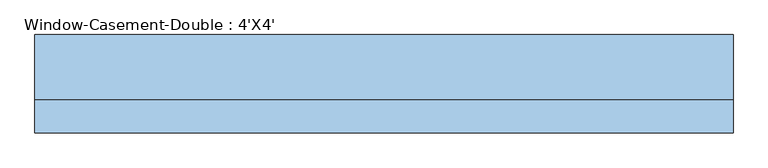
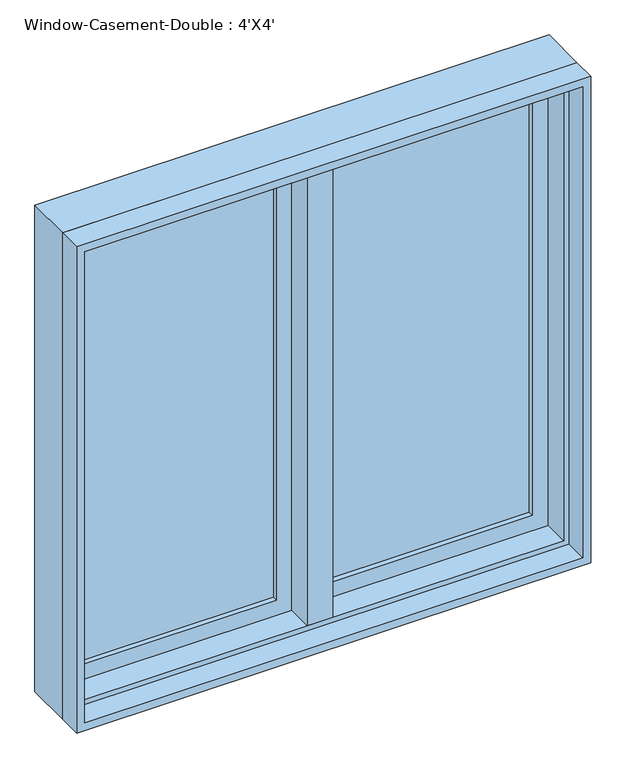
"""IFC4 building model written with IfcOpenShell, lengths in millimetres: window geometry, Window-Casement-Double : 4'X4'."""

from ifc_helpers import new_model, si_unit, frame, origin, place, context, project, spatial, polyline, outline, extrude, faceted_brep, source, transform, mapped, element, save


def window_casement_double_4_x4_191d0cfb(model_context):
    return source(origin(), model_context, "Body", "SolidModel", [
        faceted_brep([(9.525, 95.25, 2120.9), (-9.525, 95.25, 2120.9), (-9.525, 44.45, 2120.9), (9.525, 44.45, 2120.9), (9.525, 95.25, 927.1), (9.525, 44.45, 927.1), (-9.525, 44.45, 927.1), (-9.525, 95.25, 927.1), (-9.525, 44.45, 946.15), (-9.525, 44.45, 2101.85), (-30.1625, 44.45, 946.15), (-30.1625, 44.45, 2101.85), (-30.1625, -19.05, 946.15), (-30.1625, -19.05, 2101.85), (30.1625, -19.05, 946.15), (30.1625, -19.05, 2101.85), (30.1625, 44.45, 946.15), (30.1625, 44.45, 2101.85), (9.525, 44.45, 946.15), (9.525, 44.45, 2101.85)], [[[0, 1, 2, 3]], [[4, 5, 6, 7]], [[1, 0, 4, 7]], [[2, 1, 7, 6, 8, 9]], [[9, 8, 10, 11]], [[11, 10, 12, 13]], [[13, 12, 14, 15]], [[15, 14, 16, 17]], [[17, 16, 18, 19]], [[0, 3, 19, 18, 5, 4]], [[18, 8, 6, 5]], [[9, 19, 3, 2]], [[8, 18, 16, 14, 12, 10]], [[19, 9, 11, 13, 15, 17]]]),
        extrude(outline(polyline([(-66.675, 76.2), (-66.675, 69.85), (-539.75, 69.85), (-539.75, 76.2), (-66.675, 76.2)])), frame((0.0, 0.0, 984.25), z_axis=(0.0, 0.0, 1.0), x_axis=(1.0, 0.0, 0.0)), (0.0, 0.0, 1.0), 1079.5),
        extrude(outline(polyline([(-539.75, 57.15), (-539.75, 63.5), (-66.675, 63.5), (-66.675, 57.15), (-539.75, 57.15)])), frame((0.0, 0.0, 984.25), z_axis=(0.0, 0.0, 1.0), x_axis=(1.0, 0.0, 0.0)), (0.0, 0.0, 1.0), 1079.5),
        extrude(outline(polyline([(539.75, 76.2), (539.75, 69.85), (66.675, 69.85), (66.675, 76.2), (539.75, 76.2)])), frame((0.0, 0.0, 984.25), z_axis=(0.0, 0.0, 1.0), x_axis=(1.0, 0.0, 0.0)), (0.0, 0.0, 1.0), 1079.5),
        extrude(outline(polyline([(66.675, 57.15), (66.675, 63.5), (539.75, 63.5), (539.75, 57.15), (66.675, 57.15)])), frame((0.0, 0.0, 984.25), z_axis=(0.0, 0.0, 1.0), x_axis=(1.0, 0.0, 0.0)), (0.0, 0.0, 1.0), 1079.5),
        extrude(outline(polyline([(2120.9, -596.9), (927.1, -596.9), (927.1, -9.525), (2120.9, -9.525), (2120.9, -596.9)]), holes=[polyline([(2063.75, -66.675), (984.25, -66.675), (984.25, -539.75), (2063.75, -539.75), (2063.75, -66.675)])]), frame((0.0, 44.45, 0.0), z_axis=(0.0, 1.0, 0.0), x_axis=(0.0, 0.0, 1.0)), (0.0, 0.0, 1.0), 44.45),
        extrude(outline(polyline([(927.1, 596.9), (2120.9, 596.9), (2120.9, 9.525), (927.1, 9.525), (927.1, 596.9)]), holes=[polyline([(984.25, 66.675), (2063.75, 66.675), (2063.75, 539.75), (984.25, 539.75), (984.25, 66.675)])]), frame((0.0, 44.45, 0.0), z_axis=(0.0, 1.0, 0.0), x_axis=(0.0, 0.0, 1.0)), (0.0, 0.0, 1.0), 44.45),
        extrude(outline(polyline([(2133.6, -609.6), (914.4, -609.6), (914.4, 609.6), (2133.6, 609.6), (2133.6, -609.6)]), holes=[polyline([(2114.55, 590.55), (933.45, 590.55), (933.45, -590.55), (2114.55, -590.55), (2114.55, 590.55)])]), frame((0.0, -76.2, 0.0), z_axis=(0.0, 1.0, 0.0), x_axis=(0.0, 0.0, 1.0)), (0.0, 0.0, 1.0), 57.15),
        faceted_brep([(577.85, 44.45, 2101.85), (577.85, -19.05, 2101.85), (-577.85, -19.05, 2101.85), (-577.85, 44.45, 2101.85), (596.9, 95.25, 2120.9), (596.9, 44.45, 2120.9), (-596.9, 44.45, 2120.9), (-596.9, 95.25, 2120.9), (609.6, -19.05, 2133.6), (609.6, 95.25, 2133.6), (-609.6, 95.25, 2133.6), (-609.6, -19.05, 2133.6), (-577.85, -19.05, 946.15), (-577.85, 44.45, 946.15), (-596.9, 44.45, 927.1), (-596.9, 95.25, 927.1), (-609.6, 95.25, 914.4), (-609.6, -19.05, 914.4), (577.85, -19.05, 946.15), (577.85, 44.45, 946.15), (596.9, 44.45, 927.1), (596.9, 95.25, 927.1), (609.6, 95.25, 914.4), (609.6, -19.05, 914.4)], [[[0, 1, 2, 3]], [[4, 5, 6, 7]], [[8, 9, 10, 11]], [[3, 2, 12, 13]], [[7, 6, 14, 15]], [[11, 10, 16, 17]], [[13, 12, 18, 19]], [[15, 14, 20, 21]], [[17, 16, 22, 23]], [[11, 17, 23, 8], [1, 18, 12, 2]], [[19, 18, 1, 0]], [[5, 20, 14, 6], [3, 13, 19, 0]], [[21, 20, 5, 4]], [[23, 22, 9, 8]], [[9, 22, 16, 10], [7, 15, 21, 4]]]),
    ])


if __name__ == "__main__":
    model = new_model("IFC4")
    model_context = context("Model", 3, world=origin())
    ifc_project = project(units=[si_unit("LENGTHUNIT", "METRE", prefix="MILLI")], contexts=[model_context])
    site = spatial("IfcSite", under=ifc_project)
    building = spatial("IfcBuilding", under=site)
    placement = place(None, origin())
    window_casement_double_4_x4_shape = window_casement_double_4_x4_191d0cfb(model_context)
    element("IfcWindow", 1, ObjectType="Window-Casement-Double : 4'X4'", at=placement, inside=building, context=model_context, shape_type="MappedRepresentation", body=[
        mapped(window_casement_double_4_x4_shape, transform((0.0, 0.0, 0.0), x_axis=(1.0, 0.0, 0.0), y_axis=(0.0, 1.0, 0.0), z_axis=(0.0, 0.0, 1.0))),
    ])
    save(model, "model.ifc")

# Revit data of these elements
# Type "Window-Casement-Double : 4'X4'"
#   Type Mark = "19"
#   Fire Rating = "0.5h"
#   Assembly Code = "B2020100"
#   Analytic Construction = "Double glazing - domestic"
#   Frame Extension [instance default] = 0' - 0 1/4"
#   Window Inset [instance default] = 0' - 0"
#   Wall Thickness [instance default] = 0' - 6"
#   Interior Wall Closure [instance default] = 0' - 2 1/4"
#   Half Width = 2' - 0"
#   Visual Light Transmittance = 0.81
#   Thermal Resistance (R) = 1.8146 (h·ft²·°F)/BTU
#   Solar Heat Gain Coefficient = 0.76
#   Rough Width = 4' - 0 1/2"
#   Rough Height = 4' - 0 1/2"
#   Height = 4' - 0"
#   Heat Transfer Coefficient (U) = 0.5511 BTU/(h·ft²·°F)
#   Exterior Wall Closure [instance default] = 0' - 1 1/4"
#   Extension Jamb [instance default] = 0' - 2 1/4"
#   Default Sill Height = 3' - 0"
#   Width = 4' - 0"
#   Muntin Visibility = yes
#   Interior Trim Visibility [instance default] = yes
#   Exterior Trim Visibility [instance default] = yes
#   Extension Jamb Visibility [instance default] = yes
#   Interior Trim Material = Wood - Stained
#   Muntin Pattern = Muntin Pattern_2x2 : Muntin Pattern_2x2
#   Interior Trim = Trim-Window-Interior-Flat : Picture Frame
#   Interior Frame Material = Wood - Stained
#   Glass Panel Material = Glass
#   Exterior Trim Material = Clad - White
#   Exterior Trim = Trim-Window-Exterior-Flat : with Sill
#   Exterior Frame Material = Clad - White
#   Wall Closure = (empty or 0)
# Element 1 (IfcWindow, "Window-Casement-Double : 4'X4'")
#   Materials on its faces: "Wood - Stained", "Glass", "Clad - White"
# Materials
#   "Wood - Stained": class "Wood", colour RGB 224 178 126, transparency 0, Cost = 0
#   "Glass": class "Glass", colour RGB 0 128 192, transparency 0.75, Description = "Soda Lime Glass", Cost = 0
#   "Clad - White": class "Wood", colour RGB 242 242 238, transparency 0, Cost = 0
